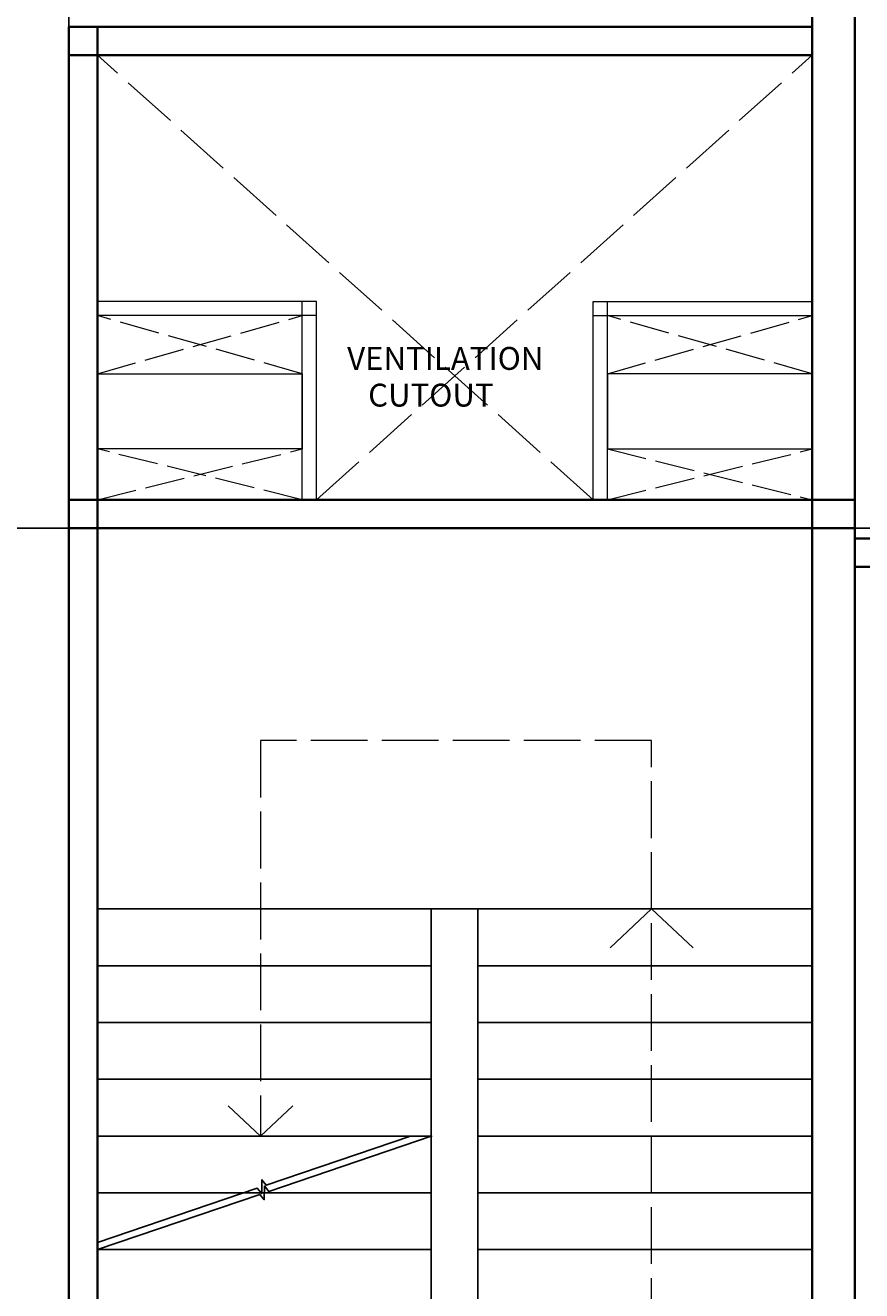
# Model space of a CAD drawing. Units: inches. Extents: x -61 to 1599, y -1316 to 257.
# Tile 190 of 204: x 826 to 1003, y -328 to -61. Entities that reach past the tile are written whole.
import ezdxf

# ---------------------------------------------------------------- set-up
doc = ezdxf.new("R2010")
doc.units = ezdxf.units.IN
doc.header["$MEASUREMENT"] = 0
doc.linetypes.add('ACAD_ISO02W100', pattern=[15, 12, -3])
for name, color, linetype, lineweight in [('A-ANNO-DIMS', 2, 'Continuous', 18), ('A-AREA-IDEN', 1, 'Continuous', 18), ('A-FLOR-OPEN', 8, 'Continuous', 18), ('A-FLOR-OPEN-HIDN', 8, 'ACAD_ISO02W100', 13), ('A-FLOR-STRS', 8, 'Continuous', 25), ('A-FLOR-STRS-PATH', 8, 'ACAD_ISO02W100', 13), ('WALLS', 4, 'Continuous', 35)]:
    doc.layers.add(name, color=color, linetype=linetype, lineweight=lineweight)
doc.styles.get("Standard").update_dxf_attribs({"font": 'arial.ttf'})
doc.dimstyles.get("Standard").update_dxf_attribs({"dimtxt": 0.18, "dimasz": 0.18, "dimexe": 0.18, "dimexo": 0.0625, "dimgap": 0.09, "dimtad": 0, "dimtih": 1, "dimtoh": 1, "dimdec": 0, "dimzin": 0, "dimdsep": 46, "dimlunit": 3, "dimtxsty": 'Standard', "dimcen": 0.09, "dimadec": 0, "dimazin": 0, "dimtfac": 1, "dimtdec": 0, "dimtofl": 0, "dimtmove": 0, "dimatfit": 3, "dimfxl": 1, "dimtolj": 1, "dimtzin": 0, "dimarcsym": 0})

# ---------------------------------------------------------------- blocks, each defined once
blk = doc.blocks.new('*D697')
at = {"layer": 'A-ANNO-DIMS', "color": 0, "lineweight": -2, "transparency": 16777216}
for p, q in [((644.7, -561.11), (644.7, 257.46)), ((644.88, 257.28), (739.94, 257.28)), ((835.52, 257.28), (740.47, 257.28)), ((835.7, -563.19), (835.7, 257.46))]:
    blk.add_line(p, q, dxfattribs=at)
at = {"layer": 'A-ANNO-DIMS', "color": 0, "transparency": 16777216}
for points in [[(644.88, 257.31), (644.88, 257.25), (644.7, 257.28)], [(835.52, 257.31), (835.52, 257.25), (835.7, 257.28)]]:
    blk.add_solid(points, dxfattribs=at)
at = {"layer": 'DEFPOINTS', "color": 0, "transparency": 16777216}
for p in [(835.7, 257.28), (644.7, -561.17), (835.7, -563.25)]:
    blk.add_point(p, dxfattribs=at)
at = {"layer": 'A-ANNO-DIMS', "color": 0, "transparency": 16777216, "insert": (740.2, 257.28), "char_height": 0.18, "attachment_point": 5}
blk.add_mtext('\\A1;191', dxfattribs=at)
blk = doc.blocks.new('*D698')
at = {"layer": 'A-ANNO-DIMS', "color": 0, "lineweight": -2, "transparency": 16777216}
for p, q in [((644.77, -167.17), (1598.48, -167.17)), ((1598.3, -167.35), (1598.3, -363.99)), ((1598.3, -560.99), (1598.3, -364.35)), ((644.77, -561.17), (1598.48, -561.17))]:
    blk.add_line(p, q, dxfattribs=at)
at = {"layer": 'A-ANNO-DIMS', "color": 0, "transparency": 16777216}
for points in [[(1598.27, -167.35), (1598.33, -167.35), (1598.3, -167.17)], [(1598.27, -560.99), (1598.33, -560.99), (1598.3, -561.17)]]:
    blk.add_solid(points, dxfattribs=at)
at = {"layer": 'DEFPOINTS', "color": 0, "transparency": 16777216}
for p in [(644.7, -167.17), (1598.3, -167.17), (644.7, -561.17)]:
    blk.add_point(p, dxfattribs=at)
at = {"layer": 'A-ANNO-DIMS', "color": 0, "transparency": 16777216, "insert": (1598.3, -364.17), "char_height": 0.18, "attachment_point": 5}
blk.add_mtext('\\A1;394', dxfattribs=at)
blk = doc.blocks.new('*D699')
at = {"layer": 'A-ANNO-DIMS', "color": 0, "lineweight": -2, "transparency": 16777216}
for p, q in [((835.64, -167.17), (-61.08, -167.17)), ((-60.9, -167.35), (-60.9, -306.73)), ((-60.9, -446.47), (-60.9, -307.09)), ((841.64, -446.65), (-61.08, -446.65))]:
    blk.add_line(p, q, dxfattribs=at)
at = {"layer": 'A-ANNO-DIMS', "color": 0, "transparency": 16777216}
for points in [[(-60.93, -167.35), (-60.87, -167.35), (-60.9, -167.17)], [(-60.93, -446.47), (-60.87, -446.47), (-60.9, -446.65)]]:
    blk.add_solid(points, dxfattribs=at)
at = {"layer": 'DEFPOINTS', "color": 0, "transparency": 16777216}
for p in [(835.7, -167.17), (-60.9, -446.65), (841.7, -446.65)]:
    blk.add_point(p, dxfattribs=at)
at = {"layer": 'A-ANNO-DIMS', "color": 0, "transparency": 16777216, "insert": (-60.9, -306.91), "char_height": 0.18, "attachment_point": 5}
blk.add_mtext('\\A1;279.5', dxfattribs=at)

msp = doc.modelspace()

# ---------------------------------------------------------------- linework, layer by layer
at = {"layer": 'A-FLOR-OPEN'}
for p, q in [((887.9857, -119.2244), (841.7028, -119.2244)), ((884.9857, -161.169), (884.9857, -119.2244)), ((887.9857, -161.169), (887.9857, -119.2244)), ((946.4198, -161.169), (946.4198, -119.2244)), ((946.4198, -119.2244), (992.7028, -119.2244)), ((949.4198, -161.169), (949.4198, -119.2244)), ((887.9857, -122.2244), (841.7028, -122.2244)), ((946.4198, -122.2244), (992.7028, -122.2244))]:
    msp.add_line(p, q, dxfattribs=at)
for points in [[(884.9857, -150.4053), (841.7028, -150.4053), (841.7028, -134.4889), (884.9857, -134.4889)], [(949.4198, -150.4053), (992.7028, -150.4053), (992.7028, -134.4889), (949.4198, -134.4889)]]:
    msp.add_lwpolyline(points, close=True, dxfattribs=at)
at = {"layer": 'A-FLOR-OPEN-HIDN'}
for p, q in [((946.4198, -161.169), (841.7028, -67.169)), ((887.9857, -161.169), (992.7028, -67.169))]:
    msp.add_line(p, q, dxfattribs=at)
at = {"layer": 'A-FLOR-OPEN-HIDN', "ltscale": 0.7}
for p, q in [((841.7028, -134.4889), (884.9857, -122.2244)), ((884.9857, -134.4889), (841.7028, -122.2244)), ((949.4198, -134.4889), (992.7028, -122.2244)), ((992.7028, -134.4889), (949.4198, -122.2244)), ((841.7028, -161.169), (884.9857, -150.4053)), ((884.9857, -161.169), (841.7028, -150.4053)), ((949.4198, -150.4053), (992.7028, -161.169)), ((949.4198, -161.169), (992.7028, -150.4053))]:
    msp.add_line(p, q, dxfattribs=at)
at = {"layer": 'A-FLOR-STRS'}
for p, q in [((992.7028, -247.6332), (841.7028, -247.6332)), ((912.2261, -247.6332), (912.2261, -367.6332)), ((922.0298, -247.6332), (922.0298, -367.6332)), ((912.2261, -259.6332), (841.7028, -259.6332)), ((992.7028, -259.6332), (922.0298, -259.6332)), ((912.2261, -271.6332), (841.7028, -271.6332)), ((992.7028, -271.6332), (922.0298, -271.6332)), ((912.2261, -283.6332), (841.7028, -283.6332)), ((992.7028, -283.6332), (922.0298, -283.6332)), ((912.2261, -295.6332), (841.7028, -295.6332)), ((992.7028, -295.6332), (922.0298, -295.6332)), ((912.2261, -307.6332), (841.7028, -307.6332)), ((992.7028, -307.6332), (922.0298, -307.6332)), ((912.2261, -319.6332), (841.7028, -319.6332)), ((992.7028, -319.6332), (922.0298, -319.6332))]:
    msp.add_line(p, q, dxfattribs=at)
for points in [[(841.7028, -319.6332), (876.0177, -307.9553), (876.9337, -309.0947), (876.9952, -306.1716), (877.9111, -307.311), (912.3965, -295.5752)], [(841.7028, -318.1486), (875.4868, -306.6515), (876.4028, -307.7909), (876.4643, -304.8677), (877.3802, -306.0071), (907.8638, -295.6332)]]:
    msp.add_lwpolyline(points, dxfattribs=at)
at = {"layer": 'A-FLOR-STRS-PATH'}
for p, q in [((958.7606, -212.0484), (876.1511, -212.0484)), ((876.1511, -212.0484), (876.1511, -295.6332)), ((958.7606, -367.6332), (958.7606, -212.0484)), ((958.7606, -247.6332), (949.4613, -256.3557)), ((958.7606, -247.6332), (968.0598, -256.3557)), ((876.1511, -295.6332), (869.3291, -289.2064)), ((876.1511, -295.6332), (882.9732, -289.2064))]:
    msp.add_line(p, q, dxfattribs=at)
at = {"layer": 'WALLS'}
for p, q in [((992.7028, 157.6771), (992.7028, -441.3229)), ((1001.7028, 157.6771), (1001.7028, -289.3229)), ((992.7028, -61.169), (992.7028, 34.831)), ((1001.7028, -169.3229), (1001.7028, -13.3229)), ((835.7028, -61.169), (835.7028, -741.169)), ((835.7028, -61.169), (992.7028, -61.169)), ((841.7028, -61.169), (841.7028, -612.169)), ((992.7028, -61.169), (992.7028, -612.169)), ((835.7028, -67.169), (992.7028, -67.169)), ((835.7028, -161.169), (1001.7028, -161.169)), ((835.7028, -167.169), (1001.7028, -167.169)), ((1001.7028, -169.3229), (1091.7028, -169.3229)), ((1001.7028, -175.3229), (1001.7028, -432.3229)), ((1001.7028, -175.3229), (1056.7028, -175.3229)), ((1001.7028, -432.3229), (1001.7028, -289.3229))]:
    msp.add_line(p, q, dxfattribs=at)

# ---------------------------------------------------------------- texts
at = {"layer": 'A-AREA-IDEN'}
for s, height, p in [('VENTILATION', 4.832098, (894.4658, -133.681)), ('   CUTOUT', 4.8321, (894.4658, -141.4434))]:
    msp.add_text(s, height=height, dxfattribs=at).set_placement(p)

# ---------------------------------------------------------------- dimensions: what is measured, and where the dimension line sits
at = {"layer": 'A-ANNO-DIMS'}
dim = msp.add_linear_dim(base=(835.7028, 257.2771), p1=(644.7028, -561.169), p2=(835.7028, -563.2524), dimstyle='Standard', override={"dimdec": 0, "dimlfac": 1, "dimrnd": 0, "dimzin": 0, "dimdsep": 46, "dimlunit": 2}, dxfattribs=at)
dim.commit()
dim.dimension.update_dxf_attribs({"geometry": '*D697', "text_midpoint": (740.2028, 257.2771)})
for base, p1, p2, override, picture, middle in [((-60.8972, -446.6462), (835.7028, -167.169), (841.7028, -446.6462), {"dimdec": 1, "dimlfac": 1, "dimrnd": 0, "dimzin": 0, "dimdsep": 46, "dimlunit": 2}, '*D699', (-60.8972, -306.9076)), ((1598.3028, -167.169), (644.7028, -561.169), (644.7028, -167.169), {"dimdec": 0, "dimlfac": 1, "dimrnd": 0, "dimzin": 0, "dimdsep": 46, "dimlunit": 2}, '*D698', (1598.3028, -364.169))]:
    dim = msp.add_linear_dim(base=base, p1=p1, p2=p2, angle=90, dimstyle='Standard', override=override, dxfattribs=at)
    dim.commit()
    dim.dimension.update_dxf_attribs({"geometry": picture, "text_midpoint": middle})

doc.saveas('drawing.dxf')
